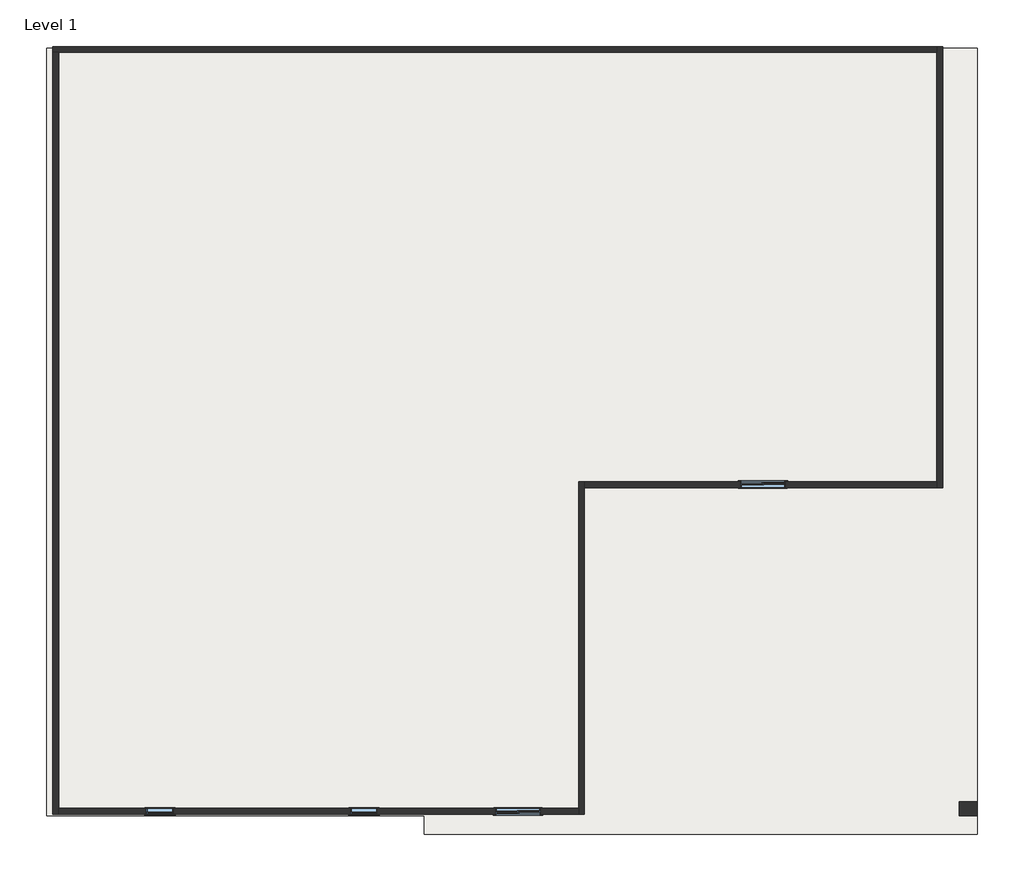
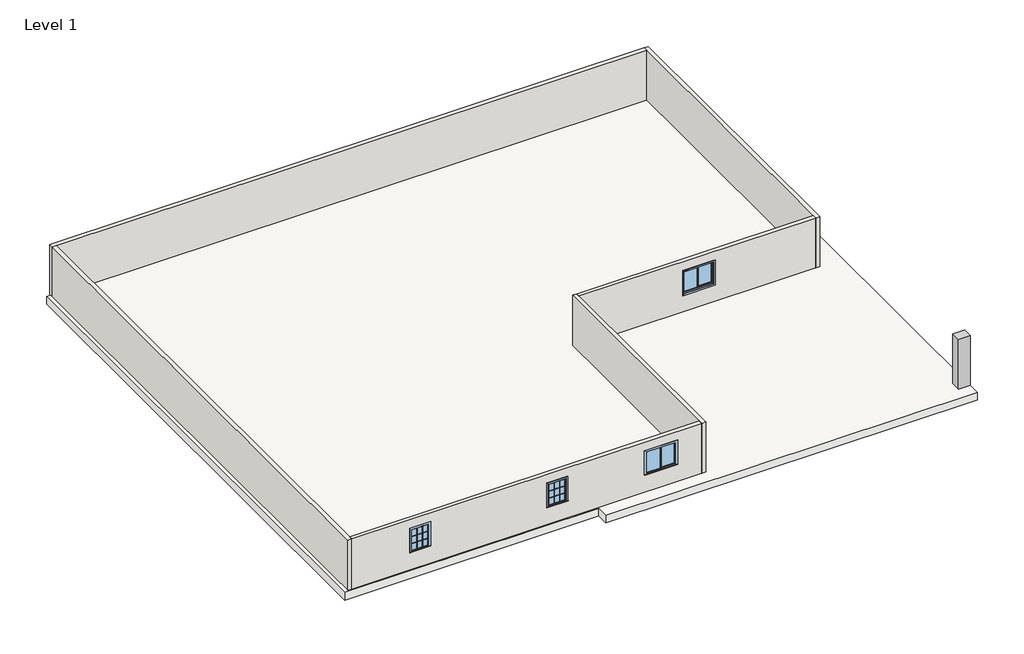
# One storey: 6 walls, 4 windows, 2 slabs, 1 column.
"""IFC4 building model written with IfcOpenShell, lengths in millimetres."""

from ifc_helpers import new_model, si_unit, frame, origin, place, context, project, spatial, polyline, outline, extrude, faceted_brep, transform, mapped, element, save
from components import m_rectangular_column_475_x_610mm_ce262976, window_ddc5d35f, window_c4d7a2b1

model = new_model("IFC4")

# Units and contexts
model_context = context("Model", 3, world=origin())
ifc_project = project(units=[si_unit("LENGTHUNIT", "METRE", prefix="MILLI")], contexts=[model_context])

# Site, building, storey
site = spatial("IfcSite", under=ifc_project)
building = spatial("IfcBuilding", under=site)
storey = spatial("IfcBuildingStorey", under=building, Name="Level 1", Elevation=2648.0)

# Column
placement = place(None, origin())
m_rectangular_column_475_x_610mm_shape = m_rectangular_column_475_x_610mm_ce262976(model_context)
element("IfcColumn", 1, ObjectType="M_Rectangular Column : 475 x 610mm", at=placement, inside=storey, context=model_context, shape_type="MappedRepresentation", body=[
    mapped(m_rectangular_column_475_x_610mm_shape, transform((9378.7171263, -7677.2043927, 0.0), x_axis=(1.0, 0.0, 0.0), y_axis=(0.0, 1.0, 0.0), z_axis=(0.0, 0.0, 1.0))),
])

# Slabs
element("IfcSlab", 2, ObjectType="Generic 5\"", at=placement, inside=storey, context=model_context, shape_type="SweptSolid", body=[
    extrude(outline(polyline([(-21609.2828737, 17887.7099289), (9680.512328, 17887.7099289), (9680.512328, -8525.0900711), (-8912.287672, -8525.0900711), (-8912.287672, -7915.4900711), (-21609.2828737, -7915.4900711), (-21609.2828737, 17887.7099289)])), frame((0.0, 0.0, 2248.0), z_axis=(0.0, 0.0, 1.0), x_axis=(1.0, 0.0, 0.0)), (0.0, 0.0, 1.0), 400.0),
])
element("IfcSlab", 3, ObjectType="Generic 5\"", at=placement, inside=storey, context=model_context, shape_type="SweptSolid", body=[
    extrude(outline(polyline([(-21609.2828737, 17887.7099289), (9680.512328, 17887.7099289), (9680.512328, -8525.0900711), (-8912.287672, -8525.0900711), (-8912.287672, -7915.4900711), (-21609.2828737, -7915.4900711), (-21609.2828737, 17887.7099289)])), frame((0.0, 0.0, 2248.0), z_axis=(0.0, 0.0, 1.0), x_axis=(1.0, 0.0, 0.0)), (0.0, 0.0, 1.0), 400.0),
])

# Walls
element("IfcWall", 4, ObjectType="Generic - 9\"", at=placement, inside=storey, context=model_context, shape_type="Brep", body=[
    faceted_brep([(-21404.4828737, 17749.7956073, 2648.0), (-21204.4828737, 17749.7956073, 2648.0), (8313.5171263, 17749.7956073, 2648.0), (8313.5171263, 17749.7956073, 5296.0), (-21204.4828737, 17749.7956073, 5296.0), (-21404.4828737, 17749.7956073, 5296.0), (-21404.4828737, 17949.7956073, 2648.0), (-21404.4828737, 17949.7956073, 5296.0), (8313.5171263, 17949.7956073, 5296.0), (8313.5171263, 17949.7956073, 2648.0)], [[[0, 1, 2, 3, 4, 5]], [[6, 7, 8, 9]], [[2, 1, 0, 6, 9]], [[5, 4, 3, 8, 7]], [[0, 5, 7, 6]], [[3, 2, 9, 8]]]),
])
element("IfcWall", 5, ObjectType="Generic - 9\"", at=placement, inside=storey, context=model_context, shape_type="Brep", body=[
    faceted_brep([(-21204.4828737, -7853.4043927, 2648.0), (-21204.4828737, -7653.4043927, 2648.0), (-21204.4828737, 17749.7956073, 2648.0), (-21204.4828737, 17749.7956073, 5296.0), (-21204.4828737, -7653.4043927, 5296.0), (-21204.4828737, -7853.4043927, 5296.0), (-21404.4828737, -7853.4043927, 2648.0), (-21404.4828737, -7853.4043927, 5296.0), (-21404.4828737, 17749.7956073, 5296.0), (-21404.4828737, 17749.7956073, 2648.0)], [[[0, 1, 2, 3, 4, 5]], [[6, 7, 8, 9]], [[2, 1, 0, 6, 9]], [[5, 4, 3, 8, 7]], [[0, 5, 7, 6]], [[3, 2, 9, 8]]]),
])
element("IfcWall", 6, ObjectType="Generic - 9\"", at=placement, inside=storey, context=model_context, shape_type="SweptSolid", body=[
    extrude(outline(polyline([(2648.0, -3726.0828737), (5296.0, -3726.0828737), (5296.0, -21204.4828737), (2648.0, -21204.4828737), (2648.0, -3726.0828737)]), holes=[polyline([(4781.6, -6521.6828737), (4781.6, -4997.6828737), (3562.4, -4997.6828737), (3562.4, -6521.6828737), (4781.6, -6521.6828737)]), polyline([(4781.6, -11398.4828737), (4781.6, -10484.0828737), (3562.4, -10484.0828737), (3562.4, -11398.4828737), (4781.6, -11398.4828737)]), polyline([(4781.6, -18256.4828737), (4781.6, -17342.0828737), (3562.4, -17342.0828737), (3562.4, -18256.4828737), (4781.6, -18256.4828737)])]), frame((0.0, -7853.4043927, 0.0), z_axis=(0.0, 1.0, 0.0), x_axis=(0.0, 0.0, 1.0)), (0.0, 0.0, 1.0), 200.0),
])
element("IfcWall", 7, ObjectType="Generic - 9\"", at=placement, inside=storey, context=model_context, shape_type="Brep", body=[
    faceted_brep([(8313.5171263, 17949.7956073, 2648.0), (8313.5171263, 17749.7956073, 2648.0), (8313.5171263, 3319.3956073, 2648.0), (8313.5171263, 3119.3956073, 2648.0), (8313.5171263, 3119.3956073, 5296.0), (8313.5171263, 3319.3956073, 5296.0), (8313.5171263, 17749.7956073, 5296.0), (8313.5171263, 17949.7956073, 5296.0), (8513.5171263, 17949.7956073, 2648.0), (8513.5171263, 17949.7956073, 5296.0), (8513.5171263, 3119.3956073, 5296.0), (8513.5171263, 3119.3956073, 2648.0)], [[[0, 1, 2, 3, 4, 5, 6, 7]], [[8, 9, 10, 11]], [[3, 2, 1, 0, 8, 11]], [[7, 6, 5, 4, 10, 9]], [[0, 7, 9, 8]], [[4, 3, 11, 10]]]),
])
element("IfcWall", 8, ObjectType="Generic - 9\"", at=placement, inside=storey, context=model_context, shape_type="Brep", body=[
    faceted_brep([(-3526.0828737, -7853.4043927, 2648.0), (-3526.0828737, 3119.3956073, 2648.0), (-3526.0828737, 3319.3956073, 2648.0), (-3526.0828737, 3319.3956073, 5296.0), (-3526.0828737, 3119.3956073, 5296.0), (-3526.0828737, -7853.4043927, 5296.0), (-3726.0828737, -7853.4043927, 2648.0), (-3726.0828737, -7853.4043927, 5296.0), (-3726.0828737, -7653.4043927, 5296.0), (-3726.0828737, 3319.3956073, 5296.0), (-3726.0828737, 3319.3956073, 2648.0), (-3726.0828737, -7653.4043927, 2648.0)], [[[0, 1, 2, 3, 4, 5]], [[6, 7, 8, 9, 10, 11]], [[2, 1, 0, 6, 11, 10]], [[5, 4, 3, 9, 8, 7]], [[3, 2, 10, 9]], [[0, 5, 7, 6]]]),
])
element("IfcWall", 9, ObjectType="Generic - 9\"", at=placement, inside=storey, context=model_context, shape_type="SweptSolid", body=[
    extrude(outline(polyline([(2648.0, -3526.0828737), (2648.0, 8313.5171263), (5296.0, 8313.5171263), (5296.0, -3526.0828737), (2648.0, -3526.0828737)]), holes=[polyline([(4781.6, 3231.9171263), (3562.4, 3231.9171263), (3562.4, 1707.9171263), (4781.6, 1707.9171263), (4781.6, 3231.9171263)])]), frame((0.0, 3119.3956073, 0.0), z_axis=(0.0, 1.0, 0.0), x_axis=(0.0, 0.0, 1.0)), (0.0, 0.0, 1.0), 200.0),
])

# Windows
window_shape = window_ddc5d35f(model_context)
element("IfcWindow", 10, ObjectType="Casement 3x3 with Trim : 36\" x 48\"", at=placement, inside=storey, context=model_context, shape_type="MappedRepresentation", body=[
    mapped(window_shape, transform((-10941.2828737, -7753.4043927, 2648.0), x_axis=(-1.0, 0.0, 0.0), y_axis=(0.0, -1.0, 0.0), z_axis=(0.0, 0.0, 1.0))),
])
element("IfcWindow", 11, ObjectType="Casement 3x3 with Trim : 36\" x 48\"", at=placement, inside=storey, context=model_context, shape_type="MappedRepresentation", body=[
    mapped(window_shape, transform((-17799.2828737, -7753.4043927, 2648.0), x_axis=(-1.0, 0.0, 0.0), y_axis=(0.0, -1.0, 0.0), z_axis=(0.0, 0.0, 1.0))),
])
window_2_shape = window_c4d7a2b1(model_context)
element("IfcWindow", 12, ObjectType="Slider with Trim : 60\" x 48\"", at=placement, inside=storey, context=model_context, shape_type="MappedRepresentation", body=[
    mapped(window_2_shape, transform((2469.9171263, 3219.3956073, 2648.0), x_axis=(1.0, 0.0, 0.0), y_axis=(0.0, 1.0, 0.0), z_axis=(0.0, 0.0, 1.0))),
])
element("IfcWindow", 13, ObjectType="Slider with Trim : 60\" x 48\"", at=placement, inside=storey, context=model_context, shape_type="MappedRepresentation", body=[
    mapped(window_2_shape, transform((-5759.6828737, -7753.4043927, 2648.0), x_axis=(-1.0, 0.0, 0.0), y_axis=(0.0, -1.0, 0.0), z_axis=(0.0, 0.0, 1.0))),
])

save(model, "model.ifc")

# Revit data of these elements
# Type "M_Rectangular Column : 475 x 610mm"
#   Depth = 1' - 6.70079"
#   Offset Base = 0' - 0"
#   Offset Top = 0' - 0"
#   Width = 2' - 0.01575"
#   Material = none
# Type "Generic 5\""
#   Function = 0
#   Layers, outside or top first: 1' - 3.74803" no material (function 1)
# Type "Generic - 9\""
#   Layers, outside or top first: 0' - 7.87402" no material (function 1)
# Type "Casement 3x3 with Trim : 36\" x 48\""
#   Type Mark = "25"
#   Construction Type Id = "GSP4R"
#   Assembly Code = "B2020100"
#   Analytic Construction = "1/8 in Pilkington single glazing"
#   Visual Light Transmittance = 0.9
#   Solar Heat Gain Coefficient = 0.78
#   Heat Transfer Coefficient (U) = 3.6886 W/(m²·K)
#   Height = 4' - 0"
#   Default Sill Height = 3' - 0"
#   Trim Projection - Ext. = 0' - 0 1/2"
#   Trim Projection - Int. = 0' - 0 3/4"
#   Trim Width - Exterior = 0' - 3 1/2"
#   Trim Width - Interior = 0' - 3 1/2"
#   Width = 3' - 0"
#   Window Inset = 0' - 0 3/4"
#   Define Thermal Properties by = 1
#   Glass Pane Material = Glass
#   Sash Material = Sash
#   Trim Exterior Material = Trim
#   Trim Interior Material = Trim
#   Wall Closure = (empty or 0)
# Type "Slider with Trim : 60\" x 48\""
#   Type Mark = "22"
#   Construction Type Id = "GSP4R"
#   Assembly Code = "B2020100"
#   Analytic Construction = "1/8 in Pilkington single glazing"
#   Visual Light Transmittance = 0.9
#   Solar Heat Gain Coefficient = 0.78
#   Heat Transfer Coefficient (U) = 3.6886 W/(m²·K)
#   Height = 4' - 0"
#   Default Sill Height = 3' - 0"
#   Trim Projection - Ext. = 0' - 0 3/4"
#   Trim Projection - Int. = 0' - 0 3/4"
#   Trim Width - Exterior = 0' - 3 1/2"
#   Trim Width - Interior = 0' - 3 1/2"
#   Width = 5' - 0"
#   Window Inset = 0' - 0 3/4"
#   Define Thermal Properties by = 1
#   Glass Pane Material = Glass
#   Sash Material = Sash
#   Trim Exterior Material = Trim
#   Trim Interior Material = Trim
#   Wall Closure = (empty or 0)
# Element 1 (IfcColumn, "M_Rectangular Column : 475 x 610mm")
#   Phase Created = New Construction
# Elements 2, 3 (IfcSlab, "Generic 5\"")
#   built-in parameter 1001955 = 3.14159 (stored number, unit not read)
#   Height Offset From Level = 0' - 0"
#   Phase Created = New Construction
#   Materials on its faces: "Default Roof"
# Elements 4, 5, 6, 7, 8, 9 (IfcWall, "Generic - 9\"")
#   Top Offset = 0' - 0"
#   Base Offset = 0' - 0"
#   Unconnected Height = 8' - 8.25197"
#   wall height = 8' - 8.25197"
#   Phase Created = New Construction
#   Base Constraint = Level 1
#   Materials on its faces: "Default Wall"
# Element 10 (IfcWindow, "Casement 3x3 with Trim : 36\" x 48\"")
#   Mark = "8"
#   Phase Created = New Construction
#   Materials on its faces: "Sash", "Glass", "Trim"
# Element 11 (IfcWindow, "Casement 3x3 with Trim : 36\" x 48\"")
#   Mark = "10"
#   Phase Created = New Construction
#   Materials on its faces: "Sash", "Glass", "Trim"
# Element 12 (IfcWindow, "Slider with Trim : 60\" x 48\"")
#   Mark = "6"
#   Phase Created = New Construction
#   Materials on its faces: "Sash", "Trim", "Glass"
# Element 13 (IfcWindow, "Slider with Trim : 60\" x 48\"")
#   Mark = "7"
#   Phase Created = New Construction
#   Materials on its faces: "Sash", "Trim", "Glass"
# Materials
#   "Glass": class "Glass", colour RGB 218 227 224, transparency 0.85, Description = "Soda Lime Glass", Cost = 0
#   "Sash": class "Wood", colour RGB 136 99 55, transparency 0
#   "Trim": class "Wood", colour RGB 224 178 126, transparency 0
#   "Default Roof": colour RGB 80 80 80, transparency 0
#   "Default Wall": colour RGB 80 80 80, transparency 0
